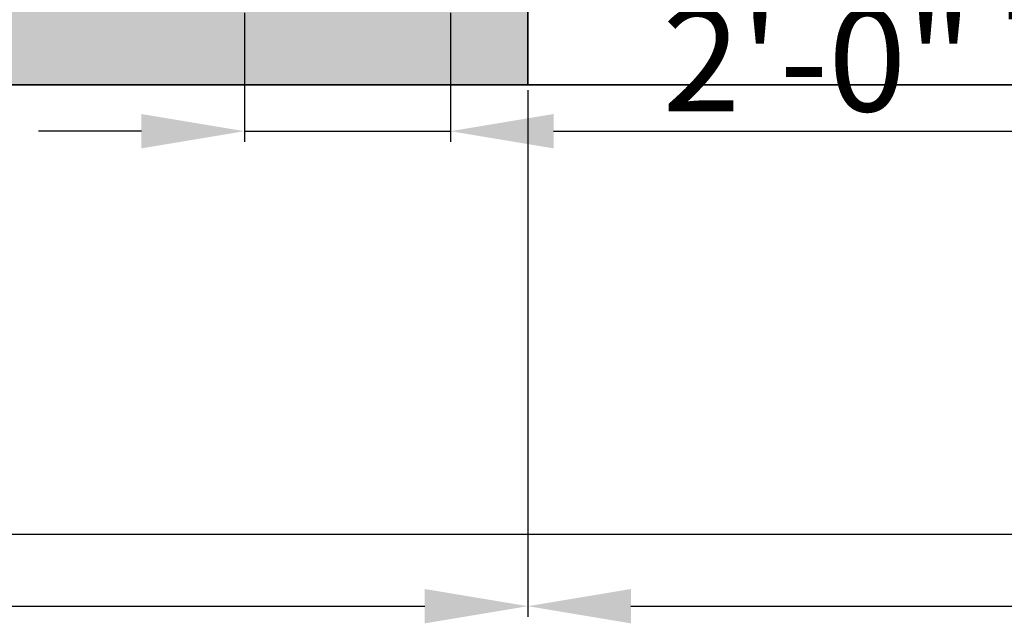
# Model space of a CAD drawing. Units: inches. Extents: x 2083 to 3317, y 1141 to 2115.
# Tile 85 of 256: x 2486 to 2600, y 1201 to 1271. Entities that reach past the tile are written whole.
import ezdxf

# ---------------------------------------------------------------- set-up
doc = ezdxf.new("R2010")
doc.units = ezdxf.units.IN
doc.layers.add('A-ANNO-DIMS', color=2, linetype='Continuous', lineweight=18)
doc.layers.add('A-WALL', color=7, linetype='Continuous', lineweight=35)
doc.layers.add('A-WALL-PATT', color=251, linetype='Continuous', lineweight=13, true_color=0x636466)
doc.styles.get("Standard").update_dxf_attribs({"font": 'arial.ttf'})
doc.dimstyles.new('ISO-25', dxfattribs={"dimtxt": 12, "dimasz": 12, "dimexe": 1.25, "dimexo": 0.625, "dimtad": 1, "dimlunit": 3, "dimtxsty": 'Standard', "dimcen": 2.5, "dimadec": 0, "dimazin": 0, "dimtfac": 1, "dimtmove": 0, "dimatfit": 3, "dimfxl": 1, "dimarcsym": 0})

# ---------------------------------------------------------------- blocks, each defined once
blk = doc.blocks.new('*D11')
at = {"layer": 'A-ANNO-DIMS', "color": 0, "lineweight": -2, "transparency": 16777216}
for p, q in [((2544.96, 1262.64), (2544.96, 1201.28)), ((2862.96, 1262.64), (2862.96, 1201.28)), ((2556.96, 1202.53), (2850.96, 1202.53))]:
    blk.add_line(p, q, dxfattribs=at)
at = {"layer": 'A-ANNO-DIMS', "color": 0, "transparency": 16777216}
for points in [[(2556.96, 1204.53), (2556.96, 1200.53), (2544.96, 1202.53)], [(2850.96, 1204.53), (2850.96, 1200.53), (2862.96, 1202.53)]]:
    blk.add_solid(points, dxfattribs=at)
at = {"layer": 'Defpoints', "color": 0, "transparency": 16777216}
for p in [(2544.96, 1263.26), (2862.96, 1263.26), (2862.96, 1202.53)]:
    blk.add_point(p, dxfattribs=at)
at = {"layer": 'A-ANNO-DIMS', "color": 0, "transparency": 16777216, "insert": (2703.96, 1209.29), "char_height": 12, "attachment_point": 5}
blk.add_mtext('26\'-6"', dxfattribs=at)
blk = doc.blocks.new('*D12')
at = {"layer": 'A-ANNO-DIMS', "color": 0, "lineweight": -2, "transparency": 16777216}
for p, q in [((2226.96, 1262.64), (2226.96, 1201.28)), ((2544.96, 1262.64), (2544.96, 1201.28)), ((2238.96, 1202.53), (2532.96, 1202.53))]:
    blk.add_line(p, q, dxfattribs=at)
at = {"layer": 'A-ANNO-DIMS', "color": 0, "transparency": 16777216}
for points in [[(2238.96, 1204.53), (2238.96, 1200.53), (2226.96, 1202.53)], [(2532.96, 1204.53), (2532.96, 1200.53), (2544.96, 1202.53)]]:
    blk.add_solid(points, dxfattribs=at)
at = {"layer": 'Defpoints', "color": 0, "transparency": 16777216}
for p in [(2226.96, 1263.26), (2544.96, 1263.26), (2544.96, 1202.53)]:
    blk.add_point(p, dxfattribs=at)
at = {"layer": 'A-ANNO-DIMS', "color": 0, "transparency": 16777216, "insert": (2385.96, 1209.29), "char_height": 12, "attachment_point": 5}
blk.add_mtext('26\'-6"', dxfattribs=at)
blk = doc.blocks.new('*D25')
at = {"layer": 'A-ANNO-DIMS', "color": 0, "lineweight": -2, "transparency": 16777216}
for p, q in [((2511.96, 1271.64), (2511.96, 1256.61)), ((2535.96, 1271.64), (2535.96, 1256.61)), ((2499.96, 1257.86), (2487.96, 1257.86)), ((2511.96, 1257.86), (2535.96, 1257.86)), ((2547.96, 1257.86), (2634.56, 1257.86))]:
    blk.add_line(p, q, dxfattribs=at)
at = {"layer": 'A-ANNO-DIMS', "color": 0, "transparency": 16777216}
for points in [[(2499.96, 1259.86), (2499.96, 1255.86), (2511.96, 1257.86)], [(2547.96, 1259.86), (2547.96, 1255.86), (2535.96, 1257.86)]]:
    blk.add_solid(points, dxfattribs=at)
at = {"layer": 'Defpoints', "color": 0, "transparency": 16777216}
for p in [(2511.96, 1272.26), (2535.96, 1272.26), (2535.96, 1257.86)]:
    blk.add_point(p, dxfattribs=at)
at = {"layer": 'A-ANNO-DIMS', "color": 0, "transparency": 16777216, "insert": (2597.26, 1264.61), "char_height": 12, "attachment_point": 5}
blk.add_mtext('2\'-0" TYP.', dxfattribs=at)
blk = doc.blocks.new('*D34')
at = {"layer": 'A-ANNO-DIMS', "color": 0, "lineweight": -2, "transparency": 16777216}
for p, q in [((2226.96, 1262.64), (2226.96, 1209.66)), ((3126.96, 1262.64), (3126.96, 1209.66)), ((2238.96, 1210.91), (3114.96, 1210.91))]:
    blk.add_line(p, q, dxfattribs=at)
at = {"layer": 'A-ANNO-DIMS', "color": 0, "transparency": 16777216}
for points in [[(2238.96, 1212.91), (2238.96, 1208.91), (2226.96, 1210.91)], [(3114.96, 1212.91), (3114.96, 1208.91), (3126.96, 1210.91)]]:
    blk.add_solid(points, dxfattribs=at)
at = {"layer": 'Defpoints', "color": 0, "transparency": 16777216}
for p in [(2226.96, 1263.26), (3126.96, 1263.26), (3126.96, 1210.91)]:
    blk.add_point(p, dxfattribs=at)
at = {"layer": 'A-ANNO-DIMS', "color": 0, "transparency": 16777216, "insert": (2676.96, 1217.66), "char_height": 12, "attachment_point": 5}
blk.add_mtext('75\'-0"', dxfattribs=at)

msp = doc.modelspace()

# ---------------------------------------------------------------- hatches: boundary and pattern name
at = {"layer": 'A-WALL-PATT'}
h = msp.add_hatch(color=256, dxfattribs=at)
h.dxf.hatch_style = 1
h.paths.add_polyline_path([(3126.96, 2020.761), (2748.96, 2020.761), (2604.96, 2020.761), (2226.96, 2020.761), (2226.96, 1702.761), (2466.96, 1702.761), (2466.96, 1582.761), (2418.96, 1582.761), (2418.96, 1477.761), (2226.96, 1477.761), (2226.96, 1263.261), (2544.96, 1263.261), (2544.96, 1411.761), (2604.96, 1411.761), (2685.96, 1411.761), (2685.96, 1420.761), (2604.96, 1420.761), (2604.96, 1573.761), (2604.96, 1702.761), (2604.96, 2011.761), (2748.96, 2011.761), (2748.96, 1702.761), (2862.96, 1702.761), (2862.96, 1621.761), (2871.96, 1621.761), (2871.96, 1702.761), (2883.96, 1702.761), (2883.96, 1706.939, -0.0264593), (2883.96, 1711.761), (2757.96, 1711.761), (2757.96, 1807.761), (2787.96, 1807.761), (2787.96, 1812.261), (2757.96, 1812.261), (2757.96, 2011.761), (2877.96, 2011.761), (2877.96, 1812.261), (2847.96, 1812.261), (2847.96, 1807.761), (2889.836, 1807.761), (2889.836, 1812.261), (2882.46, 1812.261), (2882.46, 2011.761), (3117.96, 2011.761), (3117.96, 1812.261), (2937.836, 1812.261), (2937.836, 1807.761), (2995.71, 1807.761), (2995.71, 1796.118), (3000.21, 1796.118), (3000.21, 1807.761), (3117.96, 1807.761), (3117.96, 1711.761), (3000.21, 1711.761), (3000.21, 1760.118), (2998.573, 1760.118, -0.020711), (2995.71, 1760.118), (2995.71, 1711.761), (2931.96, 1711.761), (2931.96, 1702.761), (3126.96, 1702.761)])
h.paths.add_polyline_path([(2471.46, 2011.761), (2471.46, 1810.011), (2462.717, 1810.011), (2462.717, 1805.511), (2505.96, 1805.511), (2505.96, 1810.011), (2475.96, 1810.011), (2475.96, 2011.761), (2595.96, 2011.761), (2595.96, 1810.011), (2565.96, 1810.011), (2565.96, 1805.511), (2595.96, 1805.511), (2595.96, 1711.761), (2235.96, 1711.761), (2235.96, 1805.511), (2353.71, 1805.511), (2353.71, 1796.054), (2358.21, 1796.054), (2358.21, 1805.511), (2414.717, 1805.511), (2414.717, 1810.011), (2235.96, 1810.011), (2235.96, 2011.761)], flags=16)
h.paths.add_polyline_path([(2270.205, 1994.61), (2270.205, 1970.61), (2246.205, 1970.61), (2246.205, 1994.61)], flags=0)
edge = h.paths.add_edge_path(flags=0)
edge.add_ellipse((2332.027, 1899.798), major_axis=(-3.043, 3.043), ratio=0.1682525, start_angle=-161.33217, end_angle=-156.30711, ccw=False)
edge.add_ellipse((2333.082, 1898.744), major_axis=(-1.055, 1.055), ratio=0.4535321, start_angle=-123.37102, end_angle=-94.15911)
edge = h.paths.add_edge_path(flags=0)
edge.add_ellipse((2332.027, 1968.876), major_axis=(3.043, 3.043), ratio=0.1682525, start_angle=18.66783, end_angle=23.69289)
edge.add_spline(control_points=[(2332.926, 1970.691), (2332.227, 1970.336), (2330.894, 1969.659), (2328.413, 1970.932), (2327.204, 1967.749), (2324.71, 1969.956), (2322.533, 1967.012), (2320.013, 1971.296), (2317.68, 1968.158), (2316.041, 1967.102), (2315.427, 1966.81)], knot_values=[0, 0, 0, 0, 2.2670587, 4.3245589, 6.6855835, 8.8786411, 11.121502, 14.300359, 17.7552837, 19.732645, 19.732645, 19.732645, 19.732645], degree=3, periodic=0)
edge.add_ellipse((2332.027, 1968.876), major_axis=(3.043, 3.043), ratio=0.1682525, start_angle=18.66783, end_angle=23.69289, ccw=False)
edge.add_ellipse((2333.082, 1969.931), major_axis=(1.055, 1.055), ratio=0.4535321, start_angle=56.62898, end_angle=85.84089, ccw=False)
edge = h.paths.add_edge_path(flags=0)
edge.add_spline(control_points=[(2296.428, 1967.988), (2293.628, 1965.336), (2287.704, 1959.727), (2299.744, 1949.996), (2294.533, 1935.669), (2290.573, 1920.604), (2293.394, 1909.974), (2296.185, 1904.967)], knot_values=[0.0991853, 0.0991853, 0.0991853, 0.0991853, 0.3453009, 0.6198217, 0.9826526, 1.3860932, 1.8105546, 1.8105546, 1.8105546, 1.8105546], degree=3, periodic=0)
edge.add_spline(control_points=[(2296.185, 1904.967), (2297.384, 1902.619), (2298.001, 1901.949), (2298.553, 1901.468)], knot_values=[0.0062457, 0.0062457, 0.0062457, 0.0062457, 0.0554759, 0.0554759, 0.0554759, 0.0554759], degree=3, periodic=0)
edge.add_spline(control_points=[(2298.553, 1901.468), (2297.259, 1900.923), (2295.225, 1900.232), (2293.06, 1900.614), (2292.101, 1900.788), (2292.09, 1900.791)], knot_values=[0.3128349, 0.3128349, 0.3128349, 0.3128349, 0.4017797, 0.4749867, 0.4759027, 0.4759027, 0.4759027, 0.4759027], degree=3, periodic=0)
edge.add_arc((2292.794, 1904.664), 3.937, 215.4209, 259.69818, ccw=False)
edge.add_spline(control_points=[(2289.585, 1902.382), (2289.477, 1902.535), (2289.368, 1902.688), (2289.261, 1902.841)], knot_values=[0.1028719, 0.1028719, 0.1028719, 0.1028719, 0.1168958, 0.1168958, 0.1168958, 0.1168958], degree=3, periodic=0)
edge.add_spline(control_points=[(2289.261, 1902.841), (2288.687, 1902.55), (2287.64, 1902.02), (2285.881, 1901.874), (2283.853, 1901.504), (2281.72, 1899.711), (2278.467, 1899.493), (2276.157, 1901.883), (2272.259, 1899.804), (2267.778, 1901.843), (2262.244, 1900.184), (2257.415, 1901.782), (2254.318, 1900.726), (2253.178, 1900.337)], knot_values=[0, 0, 0, 0, 1.9079767, 3.4771759, 5.261074, 7.9728515, 11.6802485, 13.7179214, 16.9395917, 22.789562, 27.5025027, 33.5952153, 37.1456181, 37.1456181, 37.1456181, 37.1456181], degree=3, periodic=0)
edge.add_line((2253.178, 1900.337), (2250.244, 1902.841))
edge.add_line((2250.244, 1902.841), (2250.244, 1965.833))
edge.add_line((2250.244, 1965.833), (2253.178, 1968.337))
edge.add_spline(control_points=[(2253.178, 1968.337), (2254.318, 1967.948), (2257.415, 1966.892), (2262.244, 1968.49), (2267.778, 1966.831), (2271.527, 1968.537), (2273.876, 1967.828), (2274.207, 1967.728)], knot_values=[0, 0, 0, 0, 0.0901802, 0.2449351, 0.3646438, 0.5132331, 0.5378548, 0.5378548, 0.5378548, 0.5378548], degree=3, periodic=0)
edge.add_arc((2274.353, 1963.793), 3.937, 72.05113, 92.12795, ccw=False)
edge.add_arc((2281.297, 1985.23), 18.596, 252.05113, 288.56572)
edge.add_arc((2292.317, 1956.029), 12.646, 71.02679, 113.77822, ccw=False)
edge = h.paths.add_edge_path(flags=0)
edge.add_spline(control_points=[(2274.899, 1951.856), (2275.066, 1951.617), (2275.233, 1951.377), (2275.398, 1951.136)], knot_values=[1.4099157, 1.4099157, 1.4099157, 1.4099157, 1.4315903, 1.4315903, 1.4315903, 1.4315903], degree=3, periodic=0)
edge.add_spline(control_points=[(2275.398, 1951.136), (2275.792, 1950.562), (2276.179, 1949.984), (2276.546, 1949.397)], knot_values=[1.3582378, 1.3582378, 1.3582378, 1.3582378, 1.4099157, 1.4099157, 1.4099157, 1.4099157], degree=3, periodic=0)
edge.add_line((2276.546, 1949.397), (2277.437, 1947.862))
edge.add_spline(control_points=[(2277.437, 1947.862), (2276.304, 1945.673), (2274.64, 1942.427), (2274.632, 1938.094), (2272.799, 1930.852), (2274.356, 1943.897), (2275.948, 1947.923), (2276.546, 1949.397)], knot_values=[0.0056315, 0.0056315, 0.0056315, 0.0056315, 0.1860139, 0.2660015, 0.3570872, 0.5963902, 0.7397317, 0.7397317, 0.7397317, 0.7397317], degree=3, periodic=0)
edge.add_spline(control_points=[(2276.546, 1949.397), (2276.179, 1949.984), (2275.792, 1950.562), (2275.398, 1951.136)], knot_values=[1.3582378, 1.3582378, 1.3582378, 1.3582378, 1.4099157, 1.4099157, 1.4099157, 1.4099157], degree=3, periodic=0)
edge.add_spline(control_points=[(2275.398, 1951.136), (2274.943, 1950.08), (2274.208, 1948.025), (2273.935, 1944.851), (2272.469, 1937.627), (2273.466, 1945.696), (2274.701, 1951.059), (2274.899, 1951.856)], knot_values=[0.1043639, 0.1043639, 0.1043639, 0.1043639, 0.1896363, 0.2696239, 0.3607096, 0.6000126, 0.6446217, 0.6446217, 0.6446217, 0.6446217], degree=3, periodic=0)
h.paths.add_polyline_path([(2269.168, 1963.128, -0.3575267), (2268.171, 1960.976, -0.0925607), (2268.171, 1939.436, -0.3575267), (2269.168, 1937.285, -0.3575267), (2267.016, 1938.282, -0.1647847), (2254.686, 1938.282, -0.3575267), (2252.534, 1937.285, -0.3575267), (2253.531, 1939.436, -0.0925607), (2253.531, 1960.976, -0.3575267), (2252.534, 1963.128, -0.3575267), (2254.686, 1962.131, -0.1647847), (2267.016, 1962.131, -0.3575267)], flags=0)
h.paths.add_polyline_path([(2248.874, 1967.802), (2248.874, 1957.028), (2249.458, 1957.028), (2249.458, 1911.647), (2248.874, 1911.647), (2248.874, 1900.873), (2246.512, 1900.873, 0.1973271), (2244.15, 1902.457), (2244.15, 1966.218, 0.1973271), (2246.512, 1967.802)], flags=0)
h.paths.add_polyline_path([(2269.168, 1931.389, -0.3575267), (2268.171, 1929.238, -0.0925607), (2268.171, 1907.698, -0.3575267), (2269.168, 1905.547, -0.3575267), (2267.016, 1906.544, -0.1647847), (2254.686, 1906.544, -0.3575267), (2252.534, 1905.547, -0.3575267), (2253.531, 1907.698, -0.0925607), (2253.531, 1929.238, -0.3575267), (2252.534, 1931.389, -0.3575267), (2254.686, 1930.392, -0.1647847), (2267.016, 1930.392, -0.3575267)], flags=0)
edge = h.paths.add_edge_path(flags=0)
edge.add_spline(control_points=[(2276.197, 1906.724), (2276.168, 1909.029), (2276.114, 1913.372), (2270.598, 1924.925), (2273.905, 1919.013), (2275.922, 1916.262), (2275.475, 1912.402), (2277.258, 1910.381), (2276.696, 1908.225), (2276.646, 1906.813), (2276.618, 1906.008)], knot_values=[0, 0, 0, 0, 8.6102597, 16.2212739, 18.8430575, 23.8048978, 27.4408283, 29.3561016, 31.2034776, 33.6506866, 33.6506866, 33.6506866, 33.6506866], degree=3, periodic=0)
edge.add_spline(control_points=[(2276.618, 1906.008), (2276.623, 1905.624), (2276.498, 1904.629), (2275.442, 1903.855), (2274.937, 1903.08), (2274.859, 1902.841)], knot_values=[0.1564884, 0.1564884, 0.1564884, 0.1564884, 0.1843975, 0.2313765, 0.2505985, 0.2505985, 0.2505985, 0.2505985], degree=3, periodic=0)
edge.add_line((2274.859, 1902.841), (2276.506, 1902.841))
edge.add_spline(control_points=[(2276.506, 1902.841), (2276.788, 1903.085), (2277.665, 1904.125), (2278.25, 1904.341), (2277.654, 1908.527), (2278.156, 1906.228), (2278.1, 1905.286), (2278.847, 1904.069), (2277.857, 1903.415), (2277.874, 1902.991), (2277.904, 1902.841)], knot_values=[0.0595743, 0.0595743, 0.0595743, 0.0595743, 0.0807529, 0.1037415, 0.1697201, 0.1760361, 0.2071372, 0.2404744, 0.2623409, 0.2736605, 0.2736605, 0.2736605, 0.2736605], degree=3, periodic=0)
edge.add_line((2277.904, 1902.841), (2280.03, 1902.841))
edge.add_spline(control_points=[(2280.03, 1902.841), (2279.888, 1903.088), (2279.499, 1903.982), (2280.152, 1905.939), (2278.104, 1909.658), (2279.762, 1907.185), (2280.328, 1904.875), (2280.485, 1903.49), (2281.463, 1903.249), (2281.758, 1902.936), (2281.834, 1902.841)], knot_values=[0.013856, 0.013856, 0.013856, 0.013856, 0.0348738, 0.0888667, 0.1078792, 0.1267378, 0.158714, 0.1937575, 0.2174868, 0.2267221, 0.2267221, 0.2267221, 0.2267221], degree=3, periodic=0)
edge.add_spline(control_points=[(2281.834, 1902.841), (2281.788, 1902.827), (2281.647, 1902.783), (2281.396, 1902.859), (2281.088, 1902.985), (2280.721, 1903.061), (2280.333, 1903.026), (2280.125, 1902.899), (2280.03, 1902.841)], knot_values=[0, 0, 0, 0, 0.1441304, 0.435517, 0.7492759, 1.1530457, 1.5483707, 1.878348, 1.878348, 1.878348, 1.878348], degree=3, periodic=0)
edge.add_line((2280.03, 1902.841), (2277.904, 1902.841))
edge.add_spline(control_points=[(2277.904, 1902.841), (2277.893, 1902.796), (2277.865, 1902.68), (2277.607, 1902.687), (2277.274, 1902.801), (2276.838, 1902.62), (2276.584, 1902.789), (2276.506, 1902.841)], knot_values=[0, 0, 0, 0, 0.1271885, 0.3261988, 0.6280094, 1.2435704, 1.5153306, 1.5153306, 1.5153306, 1.5153306], degree=3, periodic=0)
edge.add_line((2276.506, 1902.841), (2274.859, 1902.841))
edge.add_spline(control_points=[(2274.859, 1902.841), (2274.814, 1902.899), (2274.725, 1903.013), (2274.493, 1903.119), (2274.244, 1902.961), (2273.937, 1903.185), (2273.614, 1902.983), (2273.408, 1902.883), (2273.322, 1902.841)], knot_values=[0, 0, 0, 0, 0.2184302, 0.4369566, 0.6879766, 0.9903786, 1.3983955, 1.6918498, 1.6918498, 1.6918498, 1.6918498], degree=3, periodic=0)
edge.add_spline(control_points=[(2273.322, 1902.841), (2273.617, 1903.446), (2274.274, 1904.538), (2276.027, 1904.574), (2276.207, 1906.584), (2276.197, 1906.724)], knot_values=[0.0122268, 0.0122268, 0.0122268, 0.0122268, 0.0594721, 0.1062177, 0.134458, 0.134458, 0.134458, 0.134458], degree=3, periodic=0)
h.paths.add_polyline_path([(2270.776, 1897.79), (2270.776, 1873.79), (2246.776, 1873.79), (2246.776, 1897.79)], flags=0)
h.paths.add_polyline_path([(2353.71, 1760.005), (2353.71, 1760.054), (2358.21, 1760.054, -0.033729)], flags=0)
h.paths.add_polyline_path([(2321.819, 1737.529), (2341.995, 1737.529, -0.4142136), (2343.203, 1736.321), (2343.203, 1721.021, -0.4142136), (2341.995, 1719.813), (2321.819, 1719.813, -0.4142136), (2320.611, 1721.021), (2320.611, 1736.321, -0.4142136)], flags=0)
h.paths.add_polyline_path([(2324.235, 1736.321), (2339.579, 1736.321, -0.4142136), (2341.995, 1733.905), (2341.995, 1725.45, -0.4142136), (2339.579, 1723.034), (2333.681, 1723.034), (2333.845, 1722.045, -0.8706461), (2335.425, 1721.826, -0.767327), (2333.923, 1721.423), (2331.291, 1721.423, -0.767327), (2329.788, 1721.826, -0.8706461), (2331.368, 1722.045), (2331.533, 1723.034), (2324.235, 1723.034, -0.4142136), (2321.819, 1725.45), (2321.819, 1733.905, -0.4142136)], flags=0)
h.paths.add_polyline_path([(2570.484, 1928.615), (2589.684, 1928.615), (2590.169, 1928.615), (2590.169, 1904.993), (2570.484, 1904.993)], flags=0)
h.paths.add_polyline_path([(2574.447, 1927.264, -1), (2572.829, 1927.264, -1)], flags=0)
h.paths.add_polyline_path([(2573.09, 1926.941), (2573.925, 1927.776), (2574.148, 1927.553), (2573.313, 1926.718)], flags=0)
h.paths.add_polyline_path([(2578.779, 1919.73, -1), (2571.592, 1919.73, -1)], flags=0)
h.paths.add_polyline_path([(2578.385, 1919.73, -1), (2571.985, 1919.73, -1)], flags=0)
h.paths.add_polyline_path([(2331.596, 1729.476, -1), (2333.618, 1729.476, -1)], flags=0)
h.paths.add_polyline_path([(2578.034, 1927.264, -1), (2576.416, 1927.264, -1)], flags=0)
h.paths.add_polyline_path([(2576.689, 1927.531), (2576.912, 1927.754), (2577.747, 1926.919), (2577.524, 1926.696)], flags=0)
h.paths.add_polyline_path([(2578.139, 1909.86, -1), (2572.232, 1909.86, -1)], flags=0)
h.paths.add_polyline_path([(2577.745, 1909.86, -1), (2572.625, 1909.86, -1)], flags=0)
h.paths.add_polyline_path([(2583.798, 1927.264, -1), (2582.179, 1927.264, -1)], flags=0)
h.paths.add_polyline_path([(2582.719, 1927.754), (2583.554, 1926.919), (2583.331, 1926.696), (2582.496, 1927.531)], flags=0)
h.paths.add_polyline_path([(2582.496, 1927.531), (2582.719, 1927.754), (2583.554, 1926.919), (2583.331, 1926.696)], flags=0)
h.paths.add_polyline_path([(2587.739, 1920.53, -1), (2581.832, 1920.53, -1)], flags=0)
h.paths.add_polyline_path([(2587.345, 1920.53, -1), (2582.225, 1920.53, -1)], flags=0)
h.paths.add_polyline_path([(2587.385, 1927.264, -1), (2585.766, 1927.264, -1)], flags=0)
h.paths.add_polyline_path([(2586.082, 1926.98), (2586.917, 1927.815), (2587.14, 1927.593), (2586.305, 1926.758)], flags=0)
h.paths.add_polyline_path([(2588.379, 1910.66, -1), (2581.192, 1910.66, -1)], flags=0)
h.paths.add_polyline_path([(2587.985, 1910.66, -1), (2581.585, 1910.66, -1)], flags=0)
h.paths.add_polyline_path([(2417.168, 1729.478), (2437.344, 1729.478, -0.4142136), (2438.552, 1728.27), (2438.552, 1712.969, -0.4142136), (2437.344, 1711.761), (2417.168, 1711.761, -0.4142136), (2415.96, 1712.969), (2415.96, 1728.27, -0.4142136)], flags=0)
h.paths.add_polyline_path([(2419.584, 1728.27), (2434.928, 1728.27, -0.4142136), (2437.344, 1725.854), (2437.344, 1717.398, -0.4142136), (2434.928, 1714.983), (2429.029, 1714.983), (2429.194, 1713.994, -0.8706461), (2430.774, 1713.775, -0.767327), (2429.271, 1713.372), (2426.64, 1713.372, -0.767327), (2425.137, 1713.775, -0.8706461), (2426.717, 1713.994), (2426.882, 1714.983), (2419.584, 1714.983, -0.4142136), (2417.168, 1717.398), (2417.168, 1725.854, -0.4142136)], flags=0)
h.paths.add_polyline_path([(2419.584, 1728.27), (2434.928, 1728.27, -0.4142136), (2437.344, 1725.854), (2437.344, 1717.398, -0.4142136), (2434.928, 1714.983), (2429.029, 1714.983), (2428.358, 1719.009), (2427.553, 1719.009), (2426.882, 1714.983), (2419.584, 1714.983, -0.4142136), (2417.168, 1717.398), (2417.168, 1725.854, -0.4142136)], flags=0)
h.paths.add_polyline_path([(2426.944, 1721.425, -1), (2428.967, 1721.425, -1)], flags=0)
h.paths.add_polyline_path([(2475.96, 1702.761), (2595.96, 1702.761), (2595.96, 1582.761), (2475.96, 1582.761)], flags=16)
h.paths.add_polyline_path([(2427.96, 1573.761), (2595.96, 1573.761), (2595.96, 1468.761), (2595.96, 1420.761), (2384.46, 1420.761), (2384.46, 1468.761), (2427.96, 1468.761)], flags=16)
h.paths.add_polyline_path([(2379.96, 1468.761), (2379.96, 1420.761), (2235.96, 1420.761), (2235.96, 1468.761)], flags=16)
h.paths.add_polyline_path([(2317.816, 1466.696), (2337.992, 1466.696, -0.4142136), (2339.2, 1465.488), (2339.2, 1450.187, -0.4142136), (2337.992, 1448.979), (2317.816, 1448.979, -0.4142136), (2316.608, 1450.187), (2316.608, 1465.488, -0.4142136)], flags=0)
h.paths.add_polyline_path([(2320.232, 1465.488), (2335.576, 1465.488, -0.4142136), (2337.992, 1463.072), (2337.992, 1454.616, -0.4142136), (2335.576, 1452.2), (2329.677, 1452.2), (2329.842, 1451.212, -0.8706461), (2331.422, 1450.992, -0.767327), (2329.92, 1450.59), (2327.288, 1450.59, -0.767327), (2325.785, 1450.992, -0.8706461), (2327.365, 1451.212), (2327.53, 1452.2), (2320.232, 1452.2, -0.4142136), (2317.816, 1454.616), (2317.816, 1463.072, -0.4142136)], flags=0)
h.paths.add_polyline_path([(2320.232, 1465.488), (2335.576, 1465.488, -0.4142136), (2337.992, 1463.072), (2337.992, 1454.616, -0.4142136), (2335.576, 1452.2), (2329.677, 1452.2), (2329.006, 1456.227), (2328.201, 1456.227), (2327.53, 1452.2), (2320.232, 1452.2, -0.4142136), (2317.816, 1454.616), (2317.816, 1463.072, -0.4142136)], flags=0)
h.paths.add_polyline_path([(2327.593, 1458.643, -1), (2329.615, 1458.643, -1)], flags=0)
h.paths.add_polyline_path([(2244.412, 1433.34), (2241.921, 1433.34, -0.4142136), (2240.018, 1435.244), (2240.018, 1440.953, -0.4142105), (2241.921, 1442.856), (2244.412, 1442.856, -1.9764724)], flags=0)
h.paths.add_polyline_path([(2245.357, 1434.398, -0.4142136), (2245.357, 1441.799, -2.1440985)], flags=0)
h.paths.add_polyline_path([(2535.96, 1416.261), (2535.96, 1272.261), (2235.96, 1272.261), (2235.96, 1416.261)], flags=16)
h.paths.add_polyline_path([(2260.12, 1384.293), (2260.12, 1362.039), (2237.865, 1362.039), (2237.865, 1384.293)], flags=0)
edge = h.paths.add_edge_path(flags=0)
edge.add_line((2318.252, 1362.093), (2318.146, 1362.001))
edge.add_ellipse((2317.445, 1360.431), major_axis=(2.822, 2.822), ratio=0.1682525, start_angle=18.66783, end_angle=20.94813, ccw=False)
edge.add_ellipse((2318.423, 1361.409), major_axis=(0.978, 0.978), ratio=0.4535321, start_angle=56.62898, end_angle=70.2262, ccw=False)
edge = h.paths.add_edge_path(flags=0)
edge.add_line((2319.107, 1295.571), (2319.015, 1295.677))
edge.add_ellipse((2317.445, 1296.378), major_axis=(-2.822, 2.822), ratio=0.1682525, start_angle=-161.33217, end_angle=-159.05187, ccw=False)
edge.add_ellipse((2318.423, 1295.4), major_axis=(-0.978, 0.978), ratio=0.4535321, start_angle=-123.37102, end_angle=-109.7738)
edge = h.paths.add_edge_path(flags=0)
edge.add_spline(control_points=[(2284.21, 1301.17), (2284.581, 1300.445), (2284.891, 1299.892), (2285.16, 1299.461)], knot_values=[0.0390658, 0.0390658, 0.0390658, 0.0390658, 0.0554759, 0.0554759, 0.0554759, 0.0554759], degree=3, periodic=0)
edge.add_line((2285.16, 1299.461), (2284.21, 1301.17))
edge = h.paths.add_edge_path(flags=0)
edge.add_line((2280.412, 1297.298), (2283.37, 1297.036))
edge.add_line((2283.37, 1297.036), (2286.406, 1297.926))
edge.add_spline(control_points=[(2286.406, 1297.926), (2285.305, 1297.463), (2284.345, 1297.129), (2283.37, 1297.036)], knot_values=[0.3943688, 0.3943688, 0.3943688, 0.3943688, 0.4759027, 0.4759027, 0.4759027, 0.4759027], degree=3, periodic=0)
edge.add_spline(control_points=[(2283.37, 1297.036), (2283.281, 1297.028), (2282.316, 1296.957), (2281.313, 1297.134), (2280.423, 1297.296), (2280.412, 1297.298)], knot_values=[0.3128349, 0.3128349, 0.3128349, 0.3128349, 0.3202458, 0.3934528, 0.3943688, 0.3943688, 0.3943688, 0.3943688], degree=3, periodic=0)
edge = h.paths.add_edge_path(flags=0)
edge.add_line((2284.436, 1359.607), (2280.446, 1355.328))
edge.add_line((2280.446, 1355.328), (2279.58, 1351.018))
edge.add_line((2279.58, 1351.018), (2282.413, 1346.58))
edge.add_spline(control_points=[(2282.413, 1346.58), (2283.153, 1345.589), (2284.253, 1344.029), (2284.801, 1342.387), (2284.935, 1341.806)], knot_values=[1.2400982, 1.2400982, 1.2400982, 1.2400982, 1.3328922, 1.3827123, 1.3827123, 1.3827123, 1.3827123], degree=3, periodic=0)
edge.add_spline(control_points=[(2284.935, 1341.806), (2285.319, 1340.141), (2285.233, 1338.409), (2284.91, 1336.654)], knot_values=[1.0974841, 1.0974841, 1.0974841, 1.0974841, 1.2400982, 1.2400982, 1.2400982, 1.2400982], degree=3, periodic=0)
edge.add_spline(control_points=[(2284.91, 1336.654), (2284.587, 1334.899), (2284.027, 1333.12), (2283.463, 1331.361)], knot_values=[0.9548699, 0.9548699, 0.9548699, 0.9548699, 1.0974841, 1.0974841, 1.0974841, 1.0974841], degree=3, periodic=0)
edge.add_line((2283.463, 1331.361), (2281.89, 1326.153))
edge.add_line((2281.89, 1326.153), (2280.756, 1321.056))
edge.add_line((2280.756, 1321.056), (2280.299, 1316.002))
edge.add_line((2280.299, 1316.002), (2280.716, 1310.95))
edge.add_line((2280.716, 1310.95), (2282.028, 1305.972))
edge.add_line((2282.028, 1305.972), (2284.21, 1301.17))
edge.add_spline(control_points=[(2284.21, 1301.17), (2283.341, 1302.73), (2282.612, 1304.336), (2282.028, 1305.972)], knot_values=[0.0991853, 0.0991853, 0.0991853, 0.0991853, 0.2417994, 0.2417994, 0.2417994, 0.2417994], degree=3, periodic=0)
edge.add_spline(control_points=[(2282.028, 1305.972), (2281.444, 1307.608), (2281.005, 1309.273), (2280.716, 1310.95)], knot_values=[0.2417994, 0.2417994, 0.2417994, 0.2417994, 0.3844135, 0.3844135, 0.3844135, 0.3844135], degree=3, periodic=0)
edge.add_spline(control_points=[(2280.716, 1310.95), (2280.433, 1312.588), (2280.289, 1314.277), (2280.299, 1315.962), (2280.299, 1316.002)], knot_values=[0.3844135, 0.3844135, 0.3844135, 0.3844135, 0.5236467, 0.5270276, 0.5270276, 0.5270276, 0.5270276], degree=3, periodic=0)
edge.add_spline(control_points=[(2280.299, 1316.002), (2280.312, 1317.687), (2280.478, 1319.368), (2280.756, 1321.056)], knot_values=[0.5270276, 0.5270276, 0.5270276, 0.5270276, 0.6696417, 0.6696417, 0.6696417, 0.6696417], degree=3, periodic=0)
edge.add_spline(control_points=[(2280.756, 1321.056), (2281.035, 1322.744), (2281.426, 1324.44), (2281.89, 1326.153)], knot_values=[0.6696417, 0.6696417, 0.6696417, 0.6696417, 0.8122558, 0.8122558, 0.8122558, 0.8122558], degree=3, periodic=0)
edge.add_spline(control_points=[(2281.89, 1326.153), (2282.264, 1327.533), (2282.788, 1329.262), (2283.353, 1331.018), (2283.463, 1331.361)], knot_values=[0.8122558, 0.8122558, 0.8122558, 0.8122558, 0.9270873, 0.9548699, 0.9548699, 0.9548699, 0.9548699], degree=3, periodic=0)
edge.add_line((2283.463, 1331.361), (2284.91, 1336.654))
edge.add_line((2284.91, 1336.654), (2284.935, 1341.806))
edge.add_line((2284.935, 1341.806), (2282.413, 1346.58))
edge.add_spline(control_points=[(2282.413, 1346.58), (2281.275, 1348.104), (2280.078, 1349.57), (2279.58, 1351.018)], knot_values=[1.3827123, 1.3827123, 1.3827123, 1.3827123, 1.5253264, 1.5253264, 1.5253264, 1.5253264], degree=3, periodic=0)
edge.add_spline(control_points=[(2279.58, 1351.018), (2279.443, 1351.415), (2279.136, 1352.857), (2279.735, 1354.29), (2280.446, 1355.328)], knot_values=[1.5253264, 1.5253264, 1.5253264, 1.5253264, 1.564439, 1.6679405, 1.6679405, 1.6679405, 1.6679405], degree=3, periodic=0)
edge.add_spline(control_points=[(2280.446, 1355.328), (2281.426, 1356.758), (2282.931, 1358.183), (2284.436, 1359.607)], knot_values=[1.6679405, 1.6679405, 1.6679405, 1.6679405, 1.8105546, 1.8105546, 1.8105546, 1.8105546], degree=3, periodic=0)
edge.add_arc((2280.623, 1348.518), 11.726, 71.02679, 113.77822)
edge.add_arc((2270.405, 1375.595), 17.244, 252.05113, 288.56572, ccw=False)
edge.add_arc((2263.966, 1355.718), 3.651, 72.05113, 92.12795)
edge.add_arc((2263.966, 1355.718), 3.651, 92.12795, 177.98513)
edge.add_spline(control_points=[(2260.318, 1355.846), (2260.26, 1354.221), (2260.551, 1350.187), (2262.999, 1346.766), (2264.473, 1344.649)], knot_values=[1.4315903, 1.4315903, 1.4315903, 1.4315903, 1.5641438, 1.7706953, 1.7706953, 1.7706953, 1.7706953], degree=3, periodic=0)
edge.add_line((2264.473, 1344.649), (2264.936, 1343.983))
edge.add_spline(control_points=[(2263.801, 1340.248), (2263.843, 1340.514), (2264.067, 1341.756), (2264.513, 1343.002), (2264.935, 1343.981)], knot_values=[0.5365702, 0.5365702, 0.5365702, 0.5365702, 0.5593494, 0.6446217, 0.6446217, 0.6446217, 0.6446217], degree=3, periodic=0)
edge.add_spline(control_points=[(2264.935, 1343.981), (2265.118, 1343.715), (2265.299, 1343.448), (2265.477, 1343.179)], knot_values=[1.3840767, 1.3840767, 1.3840767, 1.3840767, 1.4099157, 1.4099157, 1.4099157, 1.4099157], degree=3, periodic=0)
edge.add_spline(control_points=[(2265.477, 1343.179), (2265.655, 1342.911), (2265.829, 1342.641), (2265.999, 1342.369)], knot_values=[1.3582378, 1.3582378, 1.3582378, 1.3582378, 1.3840767, 1.3840767, 1.3840767, 1.3840767], degree=3, periodic=0)
edge.add_line((2265.999, 1342.369), (2266.826, 1340.946))
edge.add_spline(control_points=[(2266.826, 1340.946), (2268.894, 1337.09), (2271.398, 1325.843), (2270.516, 1310.569), (2275.919, 1301.861), (2277.79, 1299.199)], knot_values=[0.1168958, 0.1168958, 0.1168958, 0.1168958, 0.4729873, 1.0509689, 1.3137934, 1.3137934, 1.3137934, 1.3137934], degree=3, periodic=0)
edge.add_spline(control_points=[(2277.79, 1299.199), (2277.839, 1299.128), (2277.889, 1299.057), (2277.94, 1298.987)], knot_values=[0.1098839, 0.1098839, 0.1098839, 0.1098839, 0.1168958, 0.1168958, 0.1168958, 0.1168958], degree=3, periodic=0)
edge.add_line((2277.94, 1298.987), (2277.789, 1299.199))
edge.add_spline(control_points=[(2277.789, 1299.199), (2277.257, 1298.929), (2276.286, 1298.438), (2275.039, 1298.334), (2274.383, 1298.239), (2274.215, 1298.209)], knot_values=[33.1218702, 33.1218702, 33.1218702, 33.1218702, 35.0290557, 36.5982549, 37.1448269, 37.1448269, 37.1448269, 37.1448269], degree=3, periodic=0)
edge.add_line((2274.215, 1298.209), (2273.073, 1297.893))
edge.add_spline(control_points=[(2273.073, 1297.893), (2272.323, 1297.58), (2271.039, 1296.511), (2269.248, 1296.226), (2268.423, 1296.375)], knot_values=[26.5325843, 26.5325843, 26.5325843, 26.5325843, 29.198919, 31.8391012, 31.8391012, 31.8391012, 31.8391012], degree=3, periodic=0)
edge.add_line((2268.423, 1296.375), (2263.879, 1297.458))
edge.add_spline(control_points=[(2263.879, 1297.458), (2263.556, 1297.359), (2261.86, 1296.839), (2260.239, 1297.282), (2258.933, 1297.516)], knot_values=[15.9195506, 15.9195506, 15.9195506, 15.9195506, 16.9395917, 21.2260675, 21.2260675, 21.2260675, 21.2260675], degree=3, periodic=0)
edge.add_line((2258.933, 1297.516), (2254.055, 1297.329))
edge.add_spline(control_points=[(2254.055, 1297.329), (2253.756, 1297.296), (2252.114, 1297.165), (2250.462, 1297.544), (2249.13, 1297.668)], knot_values=[5.3065169, 5.3065169, 5.3065169, 5.3065169, 6.2764352, 10.6130337, 10.6130337, 10.6130337, 10.6130337], degree=3, periodic=0)
edge.add_line((2249.13, 1297.668), (2244.332, 1296.878))
edge.add_line((2244.332, 1296.878), (2241.611, 1299.199))
edge.add_line((2241.611, 1299.199), (2241.611, 1357.609))
edge.add_line((2241.611, 1357.609), (2244.332, 1359.931))
edge.add_line((2244.332, 1359.931), (2252.729, 1359.543))
edge.add_spline(control_points=[(2252.729, 1359.543), (2252.871, 1359.546), (2253.306, 1359.548), (2253.74, 1359.514), (2254.032, 1359.482)], knot_values=[0.233291, 0.233291, 0.233291, 0.233291, 0.2449351, 0.2689274, 0.2689274, 0.2689274, 0.2689274], degree=3, periodic=0)
edge.add_line((2254.032, 1359.482), (2259.587, 1359.416))
edge.add_spline(control_points=[(2259.587, 1359.416), (2260.677, 1359.629), (2262.073, 1359.897), (2263.524, 1359.459), (2263.83, 1359.366)], knot_values=[0.4225164, 0.4225164, 0.4225164, 0.4225164, 0.5132331, 0.5378548, 0.5378548, 0.5378548, 0.5378548], degree=3, periodic=0)
edge.add_arc((2263.966, 1355.718), 3.651, 72.05113, 92.12795, ccw=False)
edge.add_arc((2270.405, 1375.595), 17.244, 252.05113, 288.56572)
edge.add_arc((2280.623, 1348.518), 11.726, 71.02679, 113.77822, ccw=False)
h.paths.add_polyline_path([(2240.341, 1359.435), (2240.341, 1349.444), (2240.882, 1349.444), (2240.882, 1307.365), (2240.341, 1307.365), (2240.341, 1297.374), (2238.15, 1297.374, 0.1973271), (2235.96, 1298.843), (2235.96, 1357.966, 0.1973271), (2238.15, 1359.435)], flags=0)
h.paths.add_polyline_path([(2259.158, 1355.101, -0.3575267), (2258.233, 1353.106, -0.0925607), (2258.233, 1333.133, -0.3575267), (2259.158, 1331.138, -0.3575267), (2257.163, 1332.062, -0.1647847), (2245.729, 1332.062, -0.3575267), (2243.735, 1331.138, -0.3575267), (2244.659, 1333.133, -0.0925607), (2244.659, 1353.106, -0.3575267), (2243.735, 1355.101, -0.3575267), (2245.729, 1354.176, -0.1647847), (2257.163, 1354.176, -0.3575267)], flags=0)
edge = h.paths.add_edge_path(flags=0)
edge.add_line((2265.999, 1342.369), (2266.826, 1340.946))
edge.add_line((2266.826, 1340.946), (2265.308, 1337.814))
edge.add_line((2265.308, 1337.814), (2264.358, 1334.653))
edge.add_line((2264.358, 1334.653), (2264.262, 1333.8))
edge.add_spline(control_points=[(2264.262, 1333.8), (2264.208, 1333.187), (2264.162, 1332.366), (2264.007, 1331.414), (2263.969, 1331.202)], knot_values=[0.4644442, 0.4644442, 0.4644442, 0.4644442, 0.5166905, 0.5316081, 0.5316081, 0.5316081, 0.5316081], degree=3, periodic=0)
edge.add_spline(control_points=[(2263.969, 1331.202), (2263.775, 1330.119), (2263.424, 1328.791), (2263.257, 1328.531), (2263.234, 1328.515)], knot_values=[0.3726816, 0.3726816, 0.3726816, 0.3726816, 0.4488497, 0.4644442, 0.4644442, 0.4644442, 0.4644442], degree=3, periodic=0)
edge.add_spline(control_points=[(2263.234, 1328.515), (2263.096, 1328.42), (2263.131, 1329.301), (2263.275, 1330.616)], knot_values=[0.2809191, 0.2809191, 0.2809191, 0.2809191, 0.3726816, 0.3726816, 0.3726816, 0.3726816], degree=3, periodic=0)
edge.add_spline(control_points=[(2263.275, 1330.616), (2263.419, 1331.93), (2263.672, 1333.677), (2263.97, 1335.315)], knot_values=[0.1891566, 0.1891566, 0.1891566, 0.1891566, 0.2809191, 0.2809191, 0.2809191, 0.2809191], degree=3, periodic=0)
edge.add_spline(control_points=[(2263.97, 1335.315), (2264.1, 1336.032), (2264.419, 1337.622), (2264.755, 1338.864), (2264.947, 1339.491)], knot_values=[0.097394, 0.097394, 0.097394, 0.097394, 0.1375775, 0.1891566, 0.1891566, 0.1891566, 0.1891566], degree=3, periodic=0)
edge.add_spline(control_points=[(2264.947, 1339.491), (2265.29, 1340.606), (2265.644, 1341.494), (2265.999, 1342.369)], knot_values=[0.0056315, 0.0056315, 0.0056315, 0.0056315, 0.097394, 0.097394, 0.097394, 0.097394], degree=3, periodic=0)
h.paths.add_polyline_path([(2259.158, 1325.671, -0.3575267), (2258.233, 1323.676, -0.0925607), (2258.233, 1303.703, -0.3575267), (2259.158, 1301.708, -0.3575267), (2257.163, 1302.633, -0.1647847), (2245.729, 1302.633, -0.3575267), (2243.735, 1301.708, -0.3575267), (2244.659, 1303.703, -0.0925607), (2244.659, 1323.676, -0.3575267), (2243.735, 1325.671, -0.3575267), (2245.729, 1324.747, -0.1647847), (2257.163, 1324.747, -0.3575267)], flags=0)
edge = h.paths.add_edge_path(flags=0)
edge.add_spline(control_points=[(2261.709, 1317.311), (2261.679, 1317.418), (2261.762, 1317.389), (2262.491, 1316.09), (2262.962, 1315.301)], knot_values=[14.9558607, 14.9558607, 14.9558607, 14.9558607, 16.2212739, 18.6948259, 18.6948259, 18.6948259, 18.6948259], degree=3, periodic=0)
edge.add_spline(control_points=[(2262.962, 1315.301), (2262.99, 1315.254), (2263.702, 1314.067), (2264.349, 1313.127), (2264.73, 1312.164)], knot_values=[18.6948259, 18.6948259, 18.6948259, 18.6948259, 18.8430575, 22.433791, 22.433791, 22.433791, 22.433791], degree=3, periodic=0)
edge.add_spline(control_points=[(2264.73, 1312.164), (2264.876, 1311.796), (2265.177, 1310.77), (2265.143, 1309.559), (2265.248, 1308.824)], knot_values=[22.433791, 22.433791, 22.433791, 22.433791, 23.8048978, 26.1727562, 26.1727562, 26.1727562, 26.1727562], degree=3, periodic=0)
edge.add_line((2265.248, 1308.824), (2265.851, 1307.172))
edge.add_spline(control_points=[(2265.851, 1307.172), (2266.065, 1306.822), (2266.384, 1306.332), (2266.424, 1305.781), (2266.42, 1305.611)], knot_values=[28.0625624, 28.0625624, 28.0625624, 28.0625624, 29.3561016, 29.9117214, 29.9117214, 29.9117214, 29.9117214], degree=3, periodic=0)
edge.add_spline(control_points=[(2266.42, 1305.611), (2266.416, 1305.433), (2266.394, 1305.25), (2266.365, 1305.066)], knot_values=[29.9117214, 29.9117214, 29.9117214, 29.9117214, 30.4978371, 30.4978371, 30.4978371, 30.4978371], degree=3, periodic=0)
edge.add_line((2266.365, 1305.066), (2266.066, 1302.136))
edge.add_spline(control_points=[(2266.066, 1302.136), (2266.071, 1301.78), (2265.998, 1301.2), (2265.663, 1300.759), (2265.509, 1300.586)], knot_values=[0.1564884, 0.1564884, 0.1564884, 0.1564884, 0.1843975, 0.2035434, 0.2035434, 0.2035434, 0.2035434], degree=3, periodic=0)
edge.add_line((2265.509, 1300.586), (2264.435, 1299.199))
edge.add_line((2264.435, 1299.199), (2265.962, 1299.199))
edge.add_line((2265.962, 1299.199), (2267.336, 1301.175))
edge.add_line((2267.336, 1301.175), (2267.312, 1301.986))
edge.add_spline(control_points=[(2267.312, 1301.986), (2267.261, 1302.862), (2267.16, 1303.737), (2267.271, 1303.326)], knot_values=[0.1262286, 0.1262286, 0.1262286, 0.1262286, 0.1666174, 0.1666174, 0.1666174, 0.1666174], degree=3, periodic=0)
edge.add_spline(control_points=[(2267.271, 1303.326), (2267.28, 1303.294), (2267.31, 1303.175), (2267.373, 1302.884), (2267.406, 1302.683), (2267.418, 1302.601)], knot_values=[0.1666174, 0.1666174, 0.1666174, 0.1666174, 0.1697201, 0.1760361, 0.1807647, 0.1807647, 0.1807647, 0.1807647], degree=3, periodic=0)
edge.add_spline(control_points=[(2267.744, 1300.988), (2267.688, 1301.151), (2267.481, 1301.657), (2267.484, 1302.145), (2267.418, 1302.601)], knot_values=[0.1807647, 0.1807647, 0.1807647, 0.1807647, 0.1937665, 0.2201389, 0.2201389, 0.2201389, 0.2201389], degree=3, periodic=0)
edge.add_line((2267.418, 1302.601), (2267.744, 1300.988))
edge.add_spline(control_points=[(2267.744, 1300.988), (2267.832, 1300.732), (2267.932, 1300.31), (2267.555, 1299.975), (2267.429, 1299.829)], knot_values=[0.2201389, 0.2201389, 0.2201389, 0.2201389, 0.2404744, 0.2548903, 0.2548903, 0.2548903, 0.2548903], degree=3, periodic=0)
edge.add_line((2267.429, 1299.829), (2267.258, 1299.199))
edge.add_line((2267.258, 1299.199), (2269.23, 1299.199))
edge.add_spline(control_points=[(2269.23, 1299.199), (2269.099, 1299.429), (2268.843, 1300.016), (2269.012, 1300.916), (2268.947, 1301.661)], knot_values=[0.013856, 0.013856, 0.013856, 0.013856, 0.0348738, 0.0670726, 0.0670726, 0.0670726, 0.0670726], degree=3, periodic=0)
edge.add_line((2268.947, 1301.661), (2268.432, 1303.603))
edge.add_spline(control_points=[(2268.432, 1303.603), (2268.176, 1304.192), (2267.596, 1305.251), (2268.041, 1304.623), (2268.251, 1304.282)], knot_values=[0.0901547, 0.0901547, 0.0901547, 0.0901547, 0.1078792, 0.1202891, 0.1202891, 0.1202891, 0.1202891], degree=3, periodic=0)
edge.add_spline(control_points=[(2268.251, 1304.282), (2268.361, 1304.105), (2269.058, 1302.918), (2269.383, 1301.59), (2269.521, 1300.776), (2269.575, 1300.556)], knot_values=[0.1202891, 0.1202891, 0.1202891, 0.1202891, 0.1267378, 0.158714, 0.1735056, 0.1735056, 0.1735056, 0.1735056], degree=3, periodic=0)
edge.add_line((2269.575, 1300.556), (2270.686, 1299.421))
edge.add_spline(control_points=[(2270.686, 1299.421), (2270.767, 1299.357), (2270.838, 1299.281), (2270.903, 1299.199)], knot_values=[0.2181597, 0.2181597, 0.2181597, 0.2181597, 0.2267221, 0.2267221, 0.2267221, 0.2267221], degree=3, periodic=0)
edge.add_line((2270.937, 1299.193), (2270.903, 1299.199))
edge.add_spline(control_points=[(2270.903, 1299.199), (2270.86, 1299.186), (2270.73, 1299.146), (2270.496, 1299.216), (2270.272, 1299.308), (2270.121, 1299.348), (2270.063, 1299.36)], knot_values=[0.939174, 0.939174, 0.939174, 0.939174, 1.0833044, 1.3746911, 1.6884499, 1.878348, 1.878348, 1.878348, 1.878348], degree=3, periodic=0)
edge.add_line((2270.063, 1299.36), (2269.23, 1299.199))
edge.add_line((2269.23, 1299.199), (2267.258, 1299.199))
edge.add_spline(control_points=[(2267.258, 1299.199), (2267.248, 1299.157), (2267.223, 1299.05), (2266.984, 1299.057), (2266.809, 1299.116), (2266.677, 1299.109), (2266.637, 1299.105)], knot_values=[0.7576653, 0.7576653, 0.7576653, 0.7576653, 0.8848538, 1.0838641, 1.3856747, 1.5153306, 1.5153306, 1.5153306, 1.5153306], degree=3, periodic=0)
edge.add_spline(control_points=[(2266.637, 1299.105), (2266.485, 1299.089), (2266.236, 1299.017), (2266.035, 1299.151), (2265.962, 1299.199)], knot_values=[0, 0, 0, 0, 0.4859051, 0.7576653, 0.7576653, 0.7576653, 0.7576653], degree=3, periodic=0)
edge.add_line((2265.962, 1299.199), (2264.435, 1299.199))
edge.add_line((2264.435, 1299.199), (2263.858, 1299.367))
edge.add_spline(control_points=[(2263.858, 1299.367), (2263.819, 1299.371), (2263.78, 1299.386), (2263.74, 1299.402)], knot_values=[0.8459249, 0.8459249, 0.8459249, 0.8459249, 0.9786272, 0.9786272, 0.9786272, 0.9786272], degree=3, periodic=0)
edge.add_line((2263.722, 1299.396), (2263.01, 1299.199))
edge.add_spline(control_points=[(2263.01, 1299.199), (2263.246, 1299.683), (2263.506, 1300.128), (2263.873, 1300.408)], knot_values=[0.0122268, 0.0122268, 0.0122268, 0.0122268, 0.0529705, 0.0529705, 0.0529705, 0.0529705], degree=3, periodic=0)
edge.add_spline(control_points=[(2263.873, 1300.408), (2263.932, 1300.453), (2264.084, 1300.553), (2264.255, 1300.624), (2264.36, 1300.665)], knot_values=[0.0529705, 0.0529705, 0.0529705, 0.0529705, 0.0594721, 0.0690861, 0.0690861, 0.0690861, 0.0690861], degree=3, periodic=0)
edge.add_line((2264.36, 1300.665), (2265.142, 1301.078))
edge.add_line((2265.142, 1301.078), (2265.676, 1302.8))
edge.add_line((2265.676, 1302.8), (2265.541, 1305.704))
edge.add_line((2265.541, 1305.704), (2264.803, 1309.328))
edge.add_line((2264.803, 1309.328), (2263.041, 1314.092))
edge.add_spline(control_points=[(2263.041, 1314.092), (2262.384, 1315.671), (2261.796, 1316.998), (2261.709, 1317.311)], knot_values=[11.2168955, 11.2168955, 11.2168955, 11.2168955, 14.9558607, 14.9558607, 14.9558607, 14.9558607], degree=3, periodic=0)
h.paths.add_polyline_path([(2871.96, 1416.261), (2895.91, 1416.261), (2895.91, 1420.761), (2871.96, 1420.761), (2871.96, 1501.761), (2862.96, 1501.761), (2862.96, 1420.761), (2805.96, 1420.761), (2805.96, 1411.761), (2862.96, 1411.761), (2862.96, 1263.261), (3126.96, 1263.261), (3126.96, 1411.761), (3126.96, 1486.761), (2943.96, 1486.761), (2943.96, 1477.761), (2967.86, 1477.761), (2967.86, 1420.761), (2943.91, 1420.761), (2943.91, 1416.261), (3117.96, 1416.261), (3117.96, 1420.761), (2972.36, 1420.761), (2972.36, 1477.761), (3117.96, 1477.761), (3117.96, 1420.761), (3117.96, 1272.261), (2871.96, 1272.261)], flags=0)
h.paths.add_polyline_path([(2457.126, 1485.943), (2527.603, 1485.943), (2527.603, 1537.636), (2457.126, 1537.636)], flags=8)
h.paths.add_polyline_path([(2481.005, 1609.982), (2590.766, 1609.982), (2590.766, 1682.003), (2481.005, 1682.003)], flags=8)
h.paths.add_polyline_path([(2483.085, 1729.127), (2553.562, 1729.127), (2553.562, 1780.82), (2483.085, 1780.82)], flags=8)

# ---------------------------------------------------------------- linework, layer by layer
at = {"layer": 'A-WALL'}
for p, q in [((2544.96, 1411.761), (2544.96, 1263.261)), ((2226.96, 1263.261), (2544.96, 1263.261)), ((2544.96, 1263.261), (3126.96, 1263.261))]:
    msp.add_line(p, q, dxfattribs=at)

# ---------------------------------------------------------------- dimensions: what is measured, and where the dimension line sits
at = {"layer": 'A-ANNO-DIMS'}
dim = msp.add_linear_dim(base=(2535.96, 1257.861), p1=(2511.96, 1272.261), p2=(2535.96, 1272.261), text='<> TYP.', dimstyle='ISO-25', override={"dimdec": 1, "dimlfac": 1, "dimrnd": 0, "dimzin": 1, "dimdsep": 46, "dimlunit": 4, "dimfrac": 2}, dxfattribs=at)
dim.commit()
dim.dimension.update_dxf_attribs({"geometry": '*D25', "text_midpoint": (2597.26, 1264.613)})
for base, p1, p2, override, picture, middle in [((2544.96, 1202.534), (2226.96, 1263.261), (2544.96, 1263.261), {"dimclrd": 0, "dimclre": 0, "dimclrt": 0}, '*D12', (2385.96, 1209.286)), ((3126.96, 1210.911), (2226.96, 1263.261), (3126.96, 1263.261), {"dimdec": 1, "dimlfac": 1, "dimrnd": 0, "dimzin": 1, "dimdsep": 46, "dimlunit": 4, "dimfrac": 2}, '*D34', (2676.96, 1217.663)), ((2862.96, 1202.534), (2544.96, 1263.261), (2862.96, 1263.261), {"dimclrd": 0, "dimclre": 0, "dimclrt": 0}, '*D11', (2703.96, 1209.286))]:
    dim = msp.add_linear_dim(base=base, p1=p1, p2=p2, dimstyle='ISO-25', override=override, dxfattribs=at)
    dim.commit()
    dim.dimension.update_dxf_attribs({"geometry": picture, "text_midpoint": middle})

doc.saveas('drawing.dxf')
